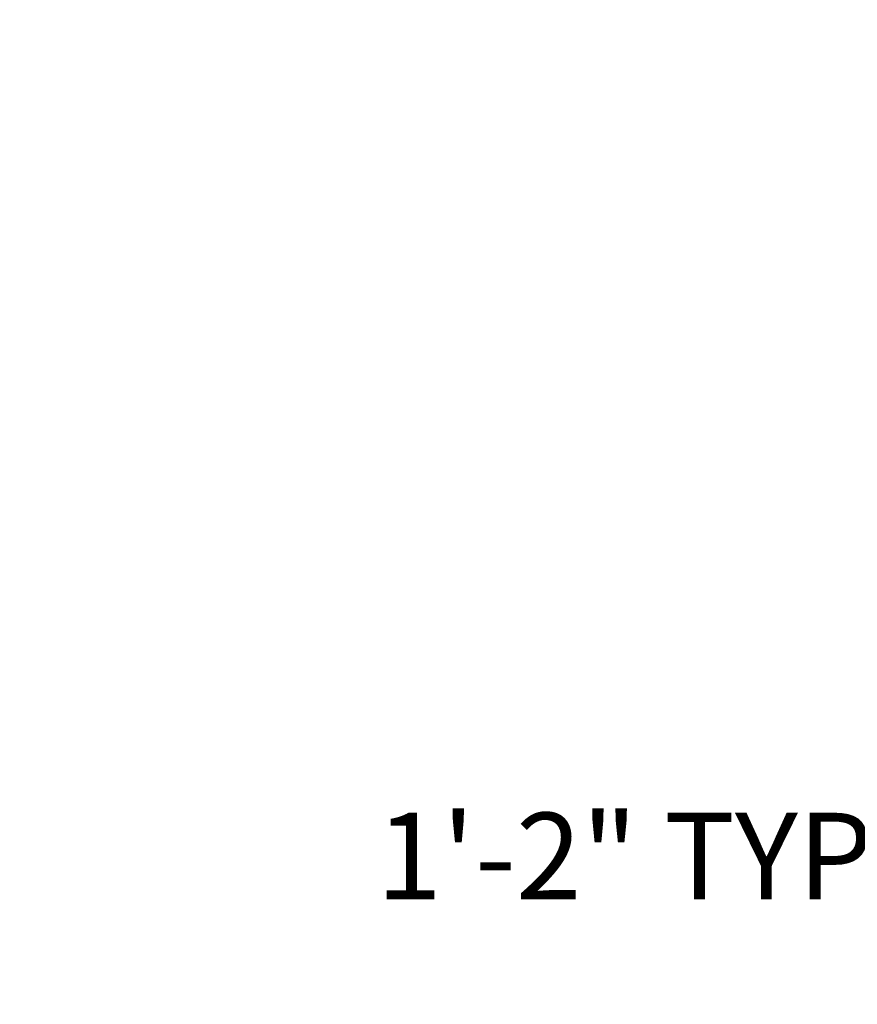
# Model space of a CAD drawing. Units: inches. Extents: x 28 to 3832, y 2 to 1709.
# Tile 2 of 7: x 2252 to 2496, y 1296 to 1582. Entities that reach past the tile are written whole.
import ezdxf

# ---------------------------------------------------------------- set-up
doc = ezdxf.new("R2010")
doc.units = ezdxf.units.IN
doc.header["$MEASUREMENT"] = 0
doc.layers.add('A-ANNO-DIMS', color=2, linetype='Continuous', lineweight=18)
doc.styles.get("Standard").update_dxf_attribs({"font": 'arial.ttf'})
doc.dimstyles.get("Standard").update_dxf_attribs({"dimtxt": 25.18, "dimasz": 20.18, "dimexe": 0.18, "dimexo": 0.0625, "dimgap": 0.09, "dimtad": 0, "dimtih": 1, "dimtoh": 1, "dimdec": 0, "dimzin": 0, "dimdsep": 46, "dimlunit": 3, "dimtxsty": 'Standard', "dimcen": 0.09, "dimadec": 0, "dimazin": 0, "dimtfac": 1, "dimtdec": 0, "dimtofl": 0, "dimtmove": 0, "dimatfit": 3, "dimfxl": 1, "dimtolj": 1, "dimtzin": 0, "dimarcsym": 0})

# ---------------------------------------------------------------- blocks, each defined once
blk = doc.blocks.new('*D24')
at = {"layer": 'A-ANNO-DIMS', "color": 0, "lineweight": -2, "transparency": 16777216}
for p, q in [((2548.85, 1347.38), (2548.85, 1338.56)), ((2562.64, 1347.38), (2562.64, 1338.56)), ((2528.67, 1338.74), (2508.49, 1338.74)), ((2582.82, 1338.74), (2603, 1338.74))]:
    blk.add_line(p, q, dxfattribs=at)
at = {"layer": 'A-ANNO-DIMS', "color": 0, "transparency": 16777216}
for points in [[(2528.67, 1342.1), (2528.67, 1335.37), (2548.85, 1338.74)], [(2582.82, 1342.1), (2582.82, 1335.37), (2562.64, 1338.74)]]:
    blk.add_solid(points, dxfattribs=at)
at = {"layer": 'Defpoints', "color": 0, "transparency": 16777216}
for p in [(2548.85, 1347.44), (2562.64, 1347.44), (2548.85, 1338.74)]:
    blk.add_point(p, dxfattribs=at)
at = {"layer": 'A-ANNO-DIMS', "color": 0, "transparency": 16777216, "insert": (2432.84, 1338.74), "char_height": 25.18, "attachment_point": 5}
blk.add_mtext('\\A1;1\'-2" TYP.', dxfattribs=at)
blk = doc.blocks.new('*D27')
at = {"layer": 'A-ANNO-DIMS', "color": 0, "lineweight": -2, "transparency": 16777216}
for p, q in [((2596.46, 1231.9), (2576.28, 1231.9)), ((2616.64, 1234.6), (2616.64, 1231.72)), ((2635.06, 1234.6), (2635.06, 1231.72)), ((2655.24, 1231.9), (2675.42, 1231.9))]:
    blk.add_line(p, q, dxfattribs=at)
at = {"layer": 'A-ANNO-DIMS', "color": 0, "transparency": 16777216}
for points in [[(2596.46, 1235.27), (2596.46, 1228.54), (2616.64, 1231.9)], [(2655.24, 1235.27), (2655.24, 1228.54), (2635.06, 1231.9)]]:
    blk.add_solid(points, dxfattribs=at)
at = {"layer": 'Defpoints', "color": 0, "transparency": 16777216}
for p in [(2616.64, 1234.67), (2616.64, 1231.9), (2635.06, 1234.67)]:
    blk.add_point(p, dxfattribs=at)
at = {"layer": 'A-ANNO-DIMS', "color": 0, "transparency": 16777216, "insert": (2410.65, 1231.9), "char_height": 25.18, "attachment_point": 5}
blk.add_mtext('\\A1;CHAIR 1\'-6 1/2" TYP.', dxfattribs=at)
blk = doc.blocks.new('*D47')
at = {"layer": 'A-ANNO-DIMS', "color": 0, "lineweight": -2, "transparency": 16777216}
for p, q in [((2562.58, 1581.52), (2507.53, 1581.52)), ((2507.71, 1561.34), (2507.71, 1255.51)), ((2507.71, 923.79), (2507.71, 1229.62)), ((2634.1, 903.61), (2507.53, 903.61))]:
    blk.add_line(p, q, dxfattribs=at)
at = {"layer": 'A-ANNO-DIMS', "color": 0, "transparency": 16777216}
for points in [[(2504.35, 1561.34), (2511.07, 1561.34), (2507.71, 1581.52)], [(2504.35, 923.79), (2511.07, 923.79), (2507.71, 903.61)]]:
    blk.add_solid(points, dxfattribs=at)
at = {"layer": 'Defpoints', "color": 0, "transparency": 16777216}
for p in [(2507.71, 1581.52), (2562.64, 1581.52), (2634.16, 903.61)]:
    blk.add_point(p, dxfattribs=at)
at = {"layer": 'A-ANNO-DIMS', "color": 0, "transparency": 16777216, "insert": (2507.71, 1242.57), "char_height": 25.18, "attachment_point": 5}
blk.add_mtext('\\A1;56\'-6"', dxfattribs=at)

msp = doc.modelspace()

# ---------------------------------------------------------------- dimensions: what is measured, and where the dimension line sits
at = {"layer": 'A-ANNO-DIMS'}
dim = msp.add_linear_dim(base=(2507.71, 1581.52), p1=(2634.16, 903.61), p2=(2562.64, 1581.52), angle=90, dimstyle='Standard', override={"dimdec": 1, "dimlfac": 1, "dimrnd": 0, "dimzin": 1, "dimdsep": 46, "dimlunit": 4, "dimfrac": 2}, dxfattribs=at)
dim.commit()
dim.dimension.update_dxf_attribs({"geometry": '*D47', "text_midpoint": (2507.71, 1242.57)})
for base, p1, p2, text, picture, middle in [((2548.85, 1338.74), (2562.64, 1347.44), (2548.85, 1347.44), '<> TYP.', '*D24', (2432.84, 1338.74)), ((2616.64, 1231.9), (2635.06, 1234.67), (2616.64, 1234.67), 'CHAIR <> TYP.', '*D27', (2410.65, 1231.9))]:
    dim = msp.add_linear_dim(base=base, p1=p1, p2=p2, angle=180, text=text, dimstyle='Standard', override={"dimdec": 1, "dimlfac": 1, "dimrnd": 0, "dimzin": 1, "dimdsep": 46, "dimlunit": 4, "dimfrac": 2}, dxfattribs=at)
    dim.commit()
    dim.dimension.update_dxf_attribs({"geometry": picture, "text_midpoint": middle})

doc.saveas('drawing.dxf')
